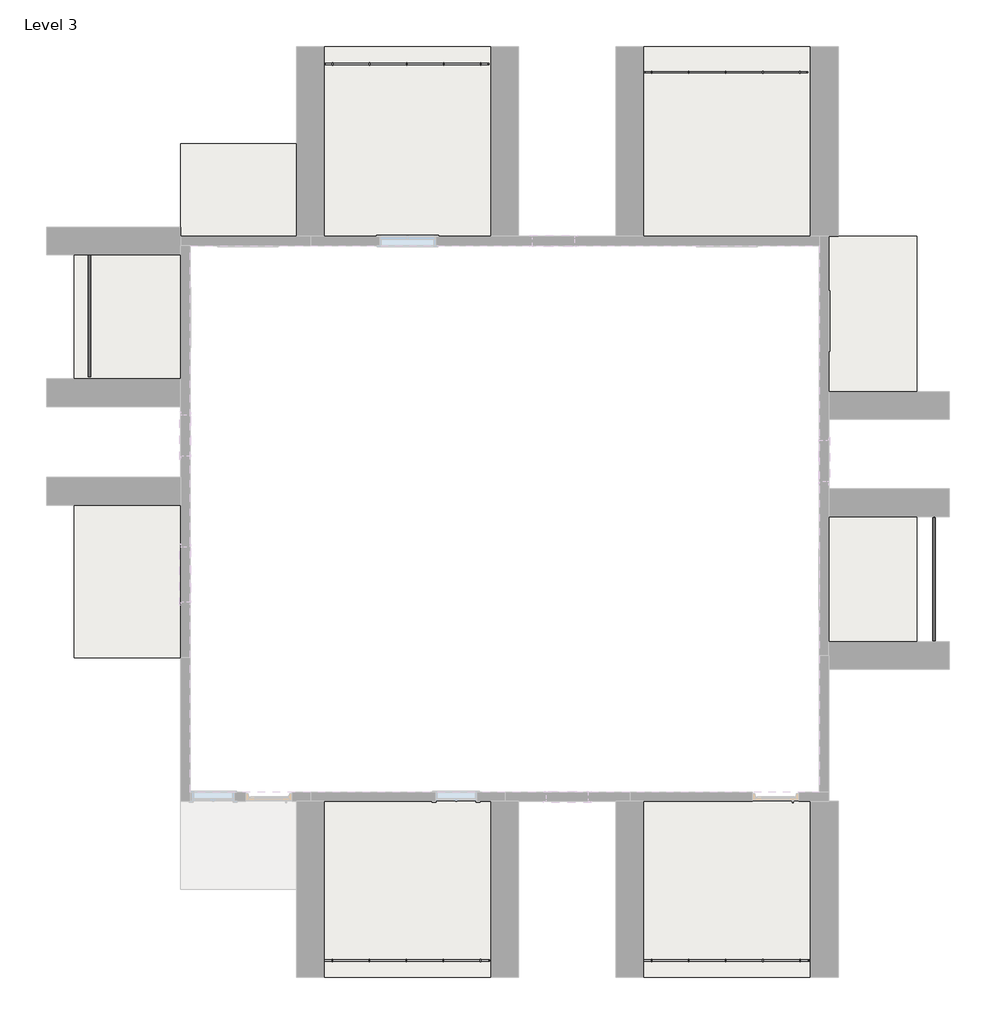
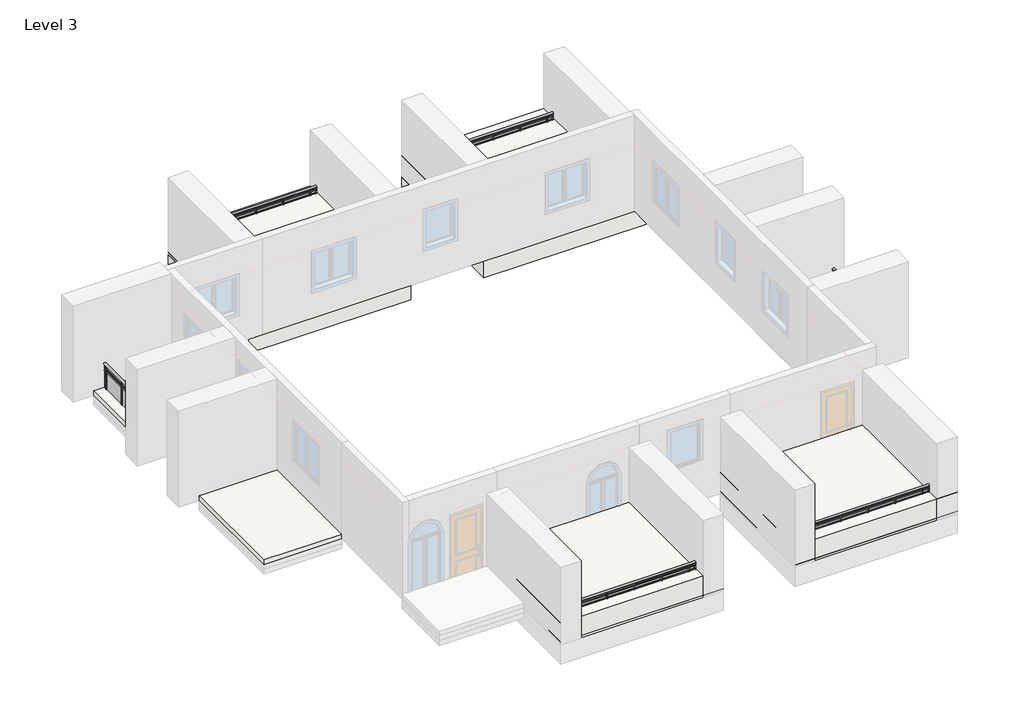
# One storey, part 2 of 2: 6 railings, 5 slabs.
"""IFC4 building model written with IfcOpenShell, lengths in millimetres."""

from ifc_helpers import new_model, si_unit, point, frame, origin, place, context, project, spatial, polyline, ellipse_curve, trimmed, outline, extrude, element, save
from ifc_brep_helpers import plane_surface, extruded_surface, advanced_brep

model = new_model("IFC4")

# Units and contexts
model_context = context("Model", 3, world=origin())
ifc_project = project(units=[si_unit("LENGTHUNIT", "METRE", prefix="MILLI")], contexts=[model_context])

# Site, building, storey
site = spatial("IfcSite", under=ifc_project)
building = spatial("IfcBuilding", under=site)
storey = spatial("IfcBuildingStorey", under=building, Name="Level 3", Elevation=6096.0)

# Railings
placement = place(None, origin())
element("IfcRailing", 1, ObjectType="Glass Panel - Bottom Fill", at=placement, inside=storey, context=model_context, shape_type="SolidModel", body=[
    advanced_brep(
    [(-9258.4937431, -9324.2034265, 7315.2), (-9258.4937431, -9400.4034265, 7315.2), (-5600.8937431, -9324.2034265, 7315.2), (-5600.8937431, -9400.4034265, 7315.2)],
    [
        (0, 1, ellipse_curve(frame((-9258.4937431, -9362.3034265, 7315.2), z_axis=(-1.0, 0.0, 0.0), x_axis=(0.0, -1.0, 0.0)), 38.1, 28.575)),
        (1, 0, ellipse_curve(frame((-9258.4937431, -9362.3034265, 7315.2), z_axis=(-1.0, 0.0, 0.0), x_axis=(0.0, -1.0, 0.0)), 38.1, 28.575)),
        (2, 3, ellipse_curve(frame((-5600.8937431, -9362.3034265, 7315.2), z_axis=(1.0, 0.0, 0.0), x_axis=(0.0, -1.0, 0.0)), 38.1, 28.575)),
        (3, 2, ellipse_curve(frame((-5600.8937431, -9362.3034265, 7315.2), z_axis=(1.0, 0.0, 0.0), x_axis=(0.0, -1.0, 0.0)), 38.1, 28.575)),
        (0, 2),
        (3, 1),
    ],
    [
        plane_surface(frame((-9258.4937431, -9362.3034265, 7315.2), z_axis=(-1.0, 0.0, 0.0), x_axis=(0.0, 1.0, 0.0))),
        plane_surface(frame((-5600.8937431, -9362.3034265, 7315.2), z_axis=(1.0, 0.0, 0.0), x_axis=(0.0, 1.0, 0.0))),
        extruded_surface(trimmed(ellipse_curve(frame((-5600.8937431, -9362.3034265, 7315.2), z_axis=(-1.0, 0.0, 0.0), x_axis=(0.0, -1.0, 0.0)), 38.1, 28.575), [point((-5600.8937431, -9324.2034265, 7315.2))], [point((-5600.8937431, -9400.4034265, 7315.2))], True, "CARTESIAN"), (-3657.5999999999995, 0.0, 0.0), 3657.5999999999995),
        extruded_surface(trimmed(ellipse_curve(frame((-5600.8937431, -9362.3034265, 7315.2), z_axis=(-1.0, 0.0, 0.0), x_axis=(0.0, -1.0, 0.0)), 38.1, 28.575), [point((-5600.8937431, -9400.4034265, 7315.2))], [point((-5600.8937431, -9324.2034265, 7315.2))], True, "CARTESIAN"), (-3657.5999999999995, 0.0, 0.0), 3657.5999999999995),
    ],
    [
        (0, [[1, 2]]),
        (1, [[3, 4]]),
        (2, [[-1, 5, -4, 6]]),
        (3, [[-2, -6, -3, -5]]),
    ],
),
    extrude(outline(polyline([(-9258.4937431, -9375.0034265), (-9258.4937431, -9349.6034265), (-5600.8937431, -9349.6034265), (-5600.8937431, -9375.0034265), (-9258.4937431, -9375.0034265)])), frame((0.0, 0.0, 7200.9), z_axis=(0.0, 0.0, 1.0), x_axis=(1.0, 0.0, 0.0)), (0.0, 0.0, 1.0), 25.4),
    extrude(outline(polyline([(-9258.4937431, -9375.0034265), (-9258.4937431, -9349.6034265), (-5600.8937431, -9349.6034265), (-5600.8937431, -9375.0034265), (-9258.4937431, -9375.0034265)])), frame((0.0, 0.0, 7099.3), z_axis=(0.0, 0.0, 1.0), x_axis=(1.0, 0.0, 0.0)), (0.0, 0.0, 1.0), 25.4),
    extrude(outline(polyline([(-5810.4437431, -9387.7034265), (-5810.4437431, -9336.9034265), (-5797.7437431, -9336.9034265), (-5797.7437431, -9387.7034265), (-5810.4437431, -9387.7034265)])), frame((0.0, 0.0, 6400.8), z_axis=(0.0, 0.0, 1.0), x_axis=(1.0, 0.0, 0.0)), (0.0, 0.0, 1.0), 885.6788223),
    extrude(outline(polyline([(-6616.8937431, -9355.7682695), (-5804.0937431, -9355.7682695), (-5804.0937431, -9362.1182695), (-6616.8937431, -9362.1182695), (-6616.8937431, -9355.7682695)])), frame((0.0, 0.0, 6502.4), z_axis=(0.0, 0.0, 1.0), x_axis=(1.0, 0.0, 0.0)), (0.0, 0.0, 1.0), 596.9),
    extrude(outline(polyline([(-6623.2437431, -9387.7034265), (-6623.2437431, -9336.9034265), (-6610.5437431, -9336.9034265), (-6610.5437431, -9387.7034265), (-6623.2437431, -9387.7034265)])), frame((0.0, 0.0, 6400.8), z_axis=(0.0, 0.0, 1.0), x_axis=(1.0, 0.0, 0.0)), (0.0, 0.0, 1.0), 885.6788223),
    extrude(outline(polyline([(-7429.6937431, -9355.7682695), (-6616.8937431, -9355.7682695), (-6616.8937431, -9362.1182695), (-7429.6937431, -9362.1182695), (-7429.6937431, -9355.7682695)])), frame((0.0, 0.0, 6502.4), z_axis=(0.0, 0.0, 1.0), x_axis=(1.0, 0.0, 0.0)), (0.0, 0.0, 1.0), 596.9),
    extrude(outline(polyline([(-7436.0437431, -9387.7034265), (-7436.0437431, -9336.9034265), (-7423.3437431, -9336.9034265), (-7423.3437431, -9387.7034265), (-7436.0437431, -9387.7034265)])), frame((0.0, 0.0, 6400.8), z_axis=(0.0, 0.0, 1.0), x_axis=(1.0, 0.0, 0.0)), (0.0, 0.0, 1.0), 885.6788223),
    extrude(outline(polyline([(-8242.4937431, -9355.7682695), (-7429.6937431, -9355.7682695), (-7429.6937431, -9362.1182695), (-8242.4937431, -9362.1182695), (-8242.4937431, -9355.7682695)])), frame((0.0, 0.0, 6502.4), z_axis=(0.0, 0.0, 1.0), x_axis=(1.0, 0.0, 0.0)), (0.0, 0.0, 1.0), 596.9),
    extrude(outline(polyline([(-8248.8437431, -9387.7034265), (-8248.8437431, -9336.9034265), (-8236.1437431, -9336.9034265), (-8236.1437431, -9387.7034265), (-8248.8437431, -9387.7034265)])), frame((0.0, 0.0, 6400.8), z_axis=(0.0, 0.0, 1.0), x_axis=(1.0, 0.0, 0.0)), (0.0, 0.0, 1.0), 885.6788223),
    extrude(outline(polyline([(-9055.2937431, -9355.7682695), (-8242.4937431, -9355.7682695), (-8242.4937431, -9362.1182695), (-9055.2937431, -9362.1182695), (-9055.2937431, -9355.7682695)])), frame((0.0, 0.0, 6502.4), z_axis=(0.0, 0.0, 1.0), x_axis=(1.0, 0.0, 0.0)), (0.0, 0.0, 1.0), 596.9),
    extrude(outline(polyline([(-9061.6437431, -9387.7034265), (-9061.6437431, -9336.9034265), (-9048.9437431, -9336.9034265), (-9048.9437431, -9387.7034265), (-9061.6437431, -9387.7034265)])), frame((0.0, 0.0, 6400.8), z_axis=(0.0, 0.0, 1.0), x_axis=(1.0, 0.0, 0.0)), (0.0, 0.0, 1.0), 885.6788223),
    extrude(outline(polyline([(-5613.5937431, -9371.8284265), (-5613.5937431, -9352.7784265), (-5594.5437431, -9352.7784265), (-5594.5437431, -9371.8284265), (-5613.5937431, -9371.8284265)])), frame((0.0, 0.0, 6400.8), z_axis=(0.0, 0.0, 1.0), x_axis=(1.0, 0.0, 0.0)), (0.0, 0.0, 1.0), 885.6788223),
    extrude(outline(polyline([(-9264.8437431, -9371.8284265), (-9264.8437431, -9352.7784265), (-9245.7937431, -9352.7784265), (-9245.7937431, -9371.8284265), (-9264.8437431, -9371.8284265)])), frame((0.0, 0.0, 6400.8), z_axis=(0.0, 0.0, 1.0), x_axis=(1.0, 0.0, 0.0)), (0.0, 0.0, 1.0), 885.6788223),
])
element("IfcRailing", 2, ObjectType="Glass Panel - Bottom Fill", at=placement, inside=storey, context=model_context, shape_type="SolidModel", body=[
    advanced_brep(
    [(-2248.0325613, -9324.2034265, 7310.1393423), (-2248.0325613, -9400.4034265, 7310.1393423), (1409.5674387, -9324.2034265, 7310.1393423), (1409.5674387, -9400.4034265, 7310.1393423)],
    [
        (0, 1, ellipse_curve(frame((-2248.0325613, -9362.3034265, 7310.1393423), z_axis=(-1.0, 0.0, 0.0), x_axis=(0.0, -1.0, 0.0)), 38.1, 28.575)),
        (1, 0, ellipse_curve(frame((-2248.0325613, -9362.3034265, 7310.1393423), z_axis=(-1.0, 0.0, 0.0), x_axis=(0.0, -1.0, 0.0)), 38.1, 28.575)),
        (2, 3, ellipse_curve(frame((1409.5674387, -9362.3034265, 7310.1393423), z_axis=(1.0, 0.0, 0.0), x_axis=(0.0, -1.0, 0.0)), 38.1, 28.575)),
        (3, 2, ellipse_curve(frame((1409.5674387, -9362.3034265, 7310.1393423), z_axis=(1.0, 0.0, 0.0), x_axis=(0.0, -1.0, 0.0)), 38.1, 28.575)),
        (0, 2),
        (3, 1),
    ],
    [
        plane_surface(frame((-2248.0325613, -9362.3034265, 7310.1393423), z_axis=(-1.0, 0.0, 0.0), x_axis=(0.0, 1.0, 0.0))),
        plane_surface(frame((1409.5674387, -9362.3034265, 7310.1393423), z_axis=(1.0, 0.0, 0.0), x_axis=(0.0, 1.0, 0.0))),
        extruded_surface(trimmed(ellipse_curve(frame((1409.5674387, -9362.3034265, 7310.1393423), z_axis=(-1.0, 0.0, 0.0), x_axis=(0.0, -1.0, 0.0)), 38.1, 28.575), [point((1409.5674387, -9324.2034265, 7310.1393423))], [point((1409.5674387, -9400.4034265, 7310.1393423))], True, "CARTESIAN"), (-3657.6, 0.0, 0.0), 3657.6),
        extruded_surface(trimmed(ellipse_curve(frame((1409.5674387, -9362.3034265, 7310.1393423), z_axis=(-1.0, 0.0, 0.0), x_axis=(0.0, -1.0, 0.0)), 38.1, 28.575), [point((1409.5674387, -9400.4034265, 7310.1393423))], [point((1409.5674387, -9324.2034265, 7310.1393423))], True, "CARTESIAN"), (-3657.6, 0.0, 0.0), 3657.6),
    ],
    [
        (0, [[1, 2]]),
        (1, [[3, 4]]),
        (2, [[-1, 5, -4, 6]]),
        (3, [[-2, -6, -3, -5]]),
    ],
),
    extrude(outline(polyline([(-2248.0325613, -9375.0034265), (-2248.0325613, -9349.6034265), (1409.5674387, -9349.6034265), (1409.5674387, -9375.0034265), (-2248.0325613, -9375.0034265)])), frame((0.0, 0.0, 7195.8393423), z_axis=(0.0, 0.0, 1.0), x_axis=(1.0, 0.0, 0.0)), (0.0, 0.0, 1.0), 25.4),
    extrude(outline(polyline([(-2248.0325613, -9375.0034265), (-2248.0325613, -9349.6034265), (1409.5674387, -9349.6034265), (1409.5674387, -9375.0034265), (-2248.0325613, -9375.0034265)])), frame((0.0, 0.0, 7094.2393423), z_axis=(0.0, 0.0, 1.0), x_axis=(1.0, 0.0, 0.0)), (0.0, 0.0, 1.0), 25.4),
    extrude(outline(polyline([(1200.0174387, -9387.7034265), (1200.0174387, -9336.9034265), (1212.7174387, -9336.9034265), (1212.7174387, -9387.7034265), (1200.0174387, -9387.7034265)])), frame((0.0, 0.0, 6395.7393423), z_axis=(0.0, 0.0, 1.0), x_axis=(1.0, 0.0, 0.0)), (0.0, 0.0, 1.0), 885.6788223),
    extrude(outline(polyline([(393.5674387, -9355.7682695), (1206.3674387, -9355.7682695), (1206.3674387, -9362.1182695), (393.5674387, -9362.1182695), (393.5674387, -9355.7682695)])), frame((0.0, 0.0, 6497.3393423), z_axis=(0.0, 0.0, 1.0), x_axis=(1.0, 0.0, 0.0)), (0.0, 0.0, 1.0), 596.9),
    extrude(outline(polyline([(387.2174387, -9387.7034265), (387.2174387, -9336.9034265), (399.9174387, -9336.9034265), (399.9174387, -9387.7034265), (387.2174387, -9387.7034265)])), frame((0.0, 0.0, 6395.7393423), z_axis=(0.0, 0.0, 1.0), x_axis=(1.0, 0.0, 0.0)), (0.0, 0.0, 1.0), 885.6788223),
    extrude(outline(polyline([(-419.2325613, -9355.7682695), (393.5674387, -9355.7682695), (393.5674387, -9362.1182695), (-419.2325613, -9362.1182695), (-419.2325613, -9355.7682695)])), frame((0.0, 0.0, 6497.3393423), z_axis=(0.0, 0.0, 1.0), x_axis=(1.0, 0.0, 0.0)), (0.0, 0.0, 1.0), 596.9),
    extrude(outline(polyline([(-425.5825613, -9387.7034265), (-425.5825613, -9336.9034265), (-412.8825613, -9336.9034265), (-412.8825613, -9387.7034265), (-425.5825613, -9387.7034265)])), frame((0.0, 0.0, 6395.7393423), z_axis=(0.0, 0.0, 1.0), x_axis=(1.0, 0.0, 0.0)), (0.0, 0.0, 1.0), 885.6788223),
    extrude(outline(polyline([(-1232.0325613, -9355.7682695), (-419.2325613, -9355.7682695), (-419.2325613, -9362.1182695), (-1232.0325613, -9362.1182695), (-1232.0325613, -9355.7682695)])), frame((0.0, 0.0, 6497.3393423), z_axis=(0.0, 0.0, 1.0), x_axis=(1.0, 0.0, 0.0)), (0.0, 0.0, 1.0), 596.9),
    extrude(outline(polyline([(-1238.3825613, -9387.7034265), (-1238.3825613, -9336.9034265), (-1225.6825613, -9336.9034265), (-1225.6825613, -9387.7034265), (-1238.3825613, -9387.7034265)])), frame((0.0, 0.0, 6395.7393423), z_axis=(0.0, 0.0, 1.0), x_axis=(1.0, 0.0, 0.0)), (0.0, 0.0, 1.0), 885.6788223),
    extrude(outline(polyline([(-2044.8325613, -9355.7682695), (-1232.0325613, -9355.7682695), (-1232.0325613, -9362.1182695), (-2044.8325613, -9362.1182695), (-2044.8325613, -9355.7682695)])), frame((0.0, 0.0, 6497.3393423), z_axis=(0.0, 0.0, 1.0), x_axis=(1.0, 0.0, 0.0)), (0.0, 0.0, 1.0), 596.9),
    extrude(outline(polyline([(-2051.1825613, -9387.7034265), (-2051.1825613, -9336.9034265), (-2038.4825613, -9336.9034265), (-2038.4825613, -9387.7034265), (-2051.1825613, -9387.7034265)])), frame((0.0, 0.0, 6395.7393423), z_axis=(0.0, 0.0, 1.0), x_axis=(1.0, 0.0, 0.0)), (0.0, 0.0, 1.0), 885.6788223),
    extrude(outline(polyline([(1396.8674387, -9371.8284265), (1396.8674387, -9352.7784265), (1415.9174387, -9352.7784265), (1415.9174387, -9371.8284265), (1396.8674387, -9371.8284265)])), frame((0.0, 0.0, 6395.7393423), z_axis=(0.0, 0.0, 1.0), x_axis=(1.0, 0.0, 0.0)), (0.0, 0.0, 1.0), 885.6788223),
    extrude(outline(polyline([(-2254.3825613, -9371.8284265), (-2254.3825613, -9352.7784265), (-2235.3325613, -9352.7784265), (-2235.3325613, -9371.8284265), (-2254.3825613, -9371.8284265)])), frame((0.0, 0.0, 6395.7393423), z_axis=(0.0, 0.0, 1.0), x_axis=(1.0, 0.0, 0.0)), (0.0, 0.0, 1.0), 885.6788223),
])
element("IfcRailing", 3, ObjectType="Glass Panel - Bottom Fill", at=placement, inside=storey, context=model_context, shape_type="SolidModel", body=[
    advanced_brep(
    [(-14351.1937431, 6115.813611, 7315.2), (-14427.3937431, 6115.813611, 7315.2), (-14351.1937431, 3448.813611, 7315.2), (-14427.3937431, 3448.813611, 7315.2)],
    [
        (0, 1, ellipse_curve(frame((-14389.2937431, 6115.813611, 7315.2), z_axis=(0.0, 1.0, 0.0), x_axis=(-1.0, 0.0, 0.0)), 38.1, 28.575)),
        (1, 0, ellipse_curve(frame((-14389.2937431, 6115.813611, 7315.2), z_axis=(0.0, 1.0, 0.0), x_axis=(-1.0, 0.0, 0.0)), 38.1, 28.575)),
        (2, 3, ellipse_curve(frame((-14389.2937431, 3448.813611, 7315.2), z_axis=(0.0, -1.0, 0.0), x_axis=(-1.0, 0.0, 0.0)), 38.1, 28.575)),
        (3, 2, ellipse_curve(frame((-14389.2937431, 3448.813611, 7315.2), z_axis=(0.0, -1.0, 0.0), x_axis=(-1.0, 0.0, 0.0)), 38.1, 28.575)),
        (0, 2),
        (3, 1),
    ],
    [
        plane_surface(frame((-14389.2937431, 6115.813611, 7315.2), z_axis=(0.0, 1.0, 0.0), x_axis=(0.0, 0.0, -1.0))),
        plane_surface(frame((-14389.2937431, 3448.813611, 7315.2), z_axis=(0.0, -1.0, 0.0), x_axis=(0.0, 0.0, -1.0))),
        extruded_surface(trimmed(ellipse_curve(frame((-14389.2937431, 3448.813611, 7315.2), z_axis=(0.0, 1.0, 0.0), x_axis=(-1.0, 0.0, 0.0)), 38.1, 28.575), [point((-14351.1937431, 3448.813611, 7315.2))], [point((-14427.3937431, 3448.813611, 7315.2))], True, "CARTESIAN"), (0.0, 2666.9999999999995, 0.0), 2666.9999999999995),
        extruded_surface(trimmed(ellipse_curve(frame((-14389.2937431, 3448.813611, 7315.2), z_axis=(0.0, 1.0, 0.0), x_axis=(-1.0, 0.0, 0.0)), 38.1, 28.575), [point((-14427.3937431, 3448.813611, 7315.2))], [point((-14351.1937431, 3448.813611, 7315.2))], True, "CARTESIAN"), (0.0, 2666.9999999999995, 0.0), 2666.9999999999995),
    ],
    [
        (0, [[1, 2]]),
        (1, [[3, 4]]),
        (2, [[-1, 5, -4, 6]]),
        (3, [[-2, -6, -3, -5]]),
    ],
),
    extrude(outline(polyline([(-14401.9937431, 6115.813611), (-14376.5937431, 6115.813611), (-14376.5937431, 3448.813611), (-14401.9937431, 3448.813611), (-14401.9937431, 6115.813611)])), frame((0.0, 0.0, 7200.9), z_axis=(0.0, 0.0, 1.0), x_axis=(1.0, 0.0, 0.0)), (0.0, 0.0, 1.0), 25.4),
    extrude(outline(polyline([(-14401.9937431, 6115.813611), (-14376.5937431, 6115.813611), (-14376.5937431, 3448.813611), (-14401.9937431, 3448.813611), (-14401.9937431, 6115.813611)])), frame((0.0, 0.0, 7099.3), z_axis=(0.0, 0.0, 1.0), x_axis=(1.0, 0.0, 0.0)), (0.0, 0.0, 1.0), 25.4),
    extrude(outline(polyline([(-14414.6937431, 3569.463611), (-14363.8937431, 3569.463611), (-14363.8937431, 3556.763611), (-14414.6937431, 3556.763611), (-14414.6937431, 3569.463611)])), frame((0.0, 0.0, 6400.8), z_axis=(0.0, 0.0, 1.0), x_axis=(1.0, 0.0, 0.0)), (0.0, 0.0, 1.0), 885.6788223),
    extrude(outline(polyline([(-14382.7585861, 4375.913611), (-14382.7585861, 3563.113611), (-14389.1085861, 3563.113611), (-14389.1085861, 4375.913611), (-14382.7585861, 4375.913611)])), frame((0.0, 0.0, 6502.4), z_axis=(0.0, 0.0, 1.0), x_axis=(1.0, 0.0, 0.0)), (0.0, 0.0, 1.0), 596.9),
    extrude(outline(polyline([(-14414.6937431, 4382.263611), (-14363.8937431, 4382.263611), (-14363.8937431, 4369.563611), (-14414.6937431, 4369.563611), (-14414.6937431, 4382.263611)])), frame((0.0, 0.0, 6400.8), z_axis=(0.0, 0.0, 1.0), x_axis=(1.0, 0.0, 0.0)), (0.0, 0.0, 1.0), 885.6788223),
    extrude(outline(polyline([(-14382.7585861, 5188.713611), (-14382.7585861, 4375.913611), (-14389.1085861, 4375.913611), (-14389.1085861, 5188.713611), (-14382.7585861, 5188.713611)])), frame((0.0, 0.0, 6502.4), z_axis=(0.0, 0.0, 1.0), x_axis=(1.0, 0.0, 0.0)), (0.0, 0.0, 1.0), 596.9),
    extrude(outline(polyline([(-14414.6937431, 5195.063611), (-14363.8937431, 5195.063611), (-14363.8937431, 5182.363611), (-14414.6937431, 5182.363611), (-14414.6937431, 5195.063611)])), frame((0.0, 0.0, 6400.8), z_axis=(0.0, 0.0, 1.0), x_axis=(1.0, 0.0, 0.0)), (0.0, 0.0, 1.0), 885.6788223),
    extrude(outline(polyline([(-14382.7585861, 6001.513611), (-14382.7585861, 5188.713611), (-14389.1085861, 5188.713611), (-14389.1085861, 6001.513611), (-14382.7585861, 6001.513611)])), frame((0.0, 0.0, 6502.4), z_axis=(0.0, 0.0, 1.0), x_axis=(1.0, 0.0, 0.0)), (0.0, 0.0, 1.0), 596.9),
    extrude(outline(polyline([(-14414.6937431, 6007.863611), (-14363.8937431, 6007.863611), (-14363.8937431, 5995.163611), (-14414.6937431, 5995.163611), (-14414.6937431, 6007.863611)])), frame((0.0, 0.0, 6400.8), z_axis=(0.0, 0.0, 1.0), x_axis=(1.0, 0.0, 0.0)), (0.0, 0.0, 1.0), 885.6788223),
    extrude(outline(polyline([(-14398.8187431, 3461.513611), (-14379.7687431, 3461.513611), (-14379.7687431, 3442.463611), (-14398.8187431, 3442.463611), (-14398.8187431, 3461.513611)])), frame((0.0, 0.0, 6400.8), z_axis=(0.0, 0.0, 1.0), x_axis=(1.0, 0.0, 0.0)), (0.0, 0.0, 1.0), 885.6788223),
    extrude(outline(polyline([(-14398.8187431, 6122.163611), (-14379.7687431, 6122.163611), (-14379.7687431, 6103.113611), (-14398.8187431, 6103.113611), (-14398.8187431, 6122.163611)])), frame((0.0, 0.0, 6400.8), z_axis=(0.0, 0.0, 1.0), x_axis=(1.0, 0.0, 0.0)), (0.0, 0.0, 1.0), 885.6788223),
])
element("IfcRailing", 4, ObjectType="Glass Panel - Bottom Fill", at=placement, inside=storey, context=model_context, shape_type="SolidModel", body=[
    advanced_brep(
    [(-9229.0758442, 10344.5205237, 7315.2), (-9229.0758442, 10268.3205237, 7315.2), (-5622.2758442, 10344.5205237, 7315.2), (-5622.2758442, 10268.3205237, 7315.2)],
    [
        (0, 1, ellipse_curve(frame((-9229.0758442, 10306.4205237, 7315.2), z_axis=(-1.0, 0.0, 0.0), x_axis=(0.0, -1.0, 0.0)), 38.1, 28.575)),
        (1, 0, ellipse_curve(frame((-9229.0758442, 10306.4205237, 7315.2), z_axis=(-1.0, 0.0, 0.0), x_axis=(0.0, -1.0, 0.0)), 38.1, 28.575)),
        (2, 3, ellipse_curve(frame((-5622.2758442, 10306.4205237, 7315.2), z_axis=(1.0, 0.0, 0.0), x_axis=(0.0, -1.0, 0.0)), 38.1, 28.575)),
        (3, 2, ellipse_curve(frame((-5622.2758442, 10306.4205237, 7315.2), z_axis=(1.0, 0.0, 0.0), x_axis=(0.0, -1.0, 0.0)), 38.1, 28.575)),
        (0, 2),
        (3, 1),
    ],
    [
        plane_surface(frame((-9229.0758442, 10306.4205237, 7315.2), z_axis=(-1.0, 0.0, 0.0), x_axis=(0.0, 1.0, 0.0))),
        plane_surface(frame((-5622.2758442, 10306.4205237, 7315.2), z_axis=(1.0, 0.0, 0.0), x_axis=(0.0, 1.0, 0.0))),
        extruded_surface(trimmed(ellipse_curve(frame((-5622.2758442, 10306.4205237, 7315.2), z_axis=(-1.0, 0.0, 0.0), x_axis=(0.0, -1.0, 0.0)), 38.1, 28.575), [point((-5622.2758442, 10344.5205237, 7315.2))], [point((-5622.2758442, 10268.3205237, 7315.2))], True, "CARTESIAN"), (-3606.8, 0.0, 0.0), 3606.8),
        extruded_surface(trimmed(ellipse_curve(frame((-5622.2758442, 10306.4205237, 7315.2), z_axis=(-1.0, 0.0, 0.0), x_axis=(0.0, -1.0, 0.0)), 38.1, 28.575), [point((-5622.2758442, 10268.3205237, 7315.2))], [point((-5622.2758442, 10344.5205237, 7315.2))], True, "CARTESIAN"), (-3606.8, 0.0, 0.0), 3606.8),
    ],
    [
        (0, [[1, 2]]),
        (1, [[3, 4]]),
        (2, [[-1, 5, -4, 6]]),
        (3, [[-2, -6, -3, -5]]),
    ],
),
    extrude(outline(polyline([(-9229.0758442, 10293.7205237), (-9229.0758442, 10319.1205237), (-5622.2758442, 10319.1205237), (-5622.2758442, 10293.7205237), (-9229.0758442, 10293.7205237)])), frame((0.0, 0.0, 7200.9), z_axis=(0.0, 0.0, 1.0), x_axis=(1.0, 0.0, 0.0)), (0.0, 0.0, 1.0), 25.4),
    extrude(outline(polyline([(-9229.0758442, 10293.7205237), (-9229.0758442, 10319.1205237), (-5622.2758442, 10319.1205237), (-5622.2758442, 10293.7205237), (-9229.0758442, 10293.7205237)])), frame((0.0, 0.0, 7099.3), z_axis=(0.0, 0.0, 1.0), x_axis=(1.0, 0.0, 0.0)), (0.0, 0.0, 1.0), 25.4),
    extrude(outline(polyline([(-5806.4258442, 10281.0205237), (-5806.4258442, 10331.8205237), (-5793.7258442, 10331.8205237), (-5793.7258442, 10281.0205237), (-5806.4258442, 10281.0205237)])), frame((0.0, 0.0, 6400.8), z_axis=(0.0, 0.0, 1.0), x_axis=(1.0, 0.0, 0.0)), (0.0, 0.0, 1.0), 885.6788223),
    extrude(outline(polyline([(-6612.8758442, 10312.9556807), (-5800.0758442, 10312.9556807), (-5800.0758442, 10306.6056807), (-6612.8758442, 10306.6056807), (-6612.8758442, 10312.9556807)])), frame((0.0, 0.0, 6502.4), z_axis=(0.0, 0.0, 1.0), x_axis=(1.0, 0.0, 0.0)), (0.0, 0.0, 1.0), 596.9),
    extrude(outline(polyline([(-6619.2258442, 10281.0205237), (-6619.2258442, 10331.8205237), (-6606.5258442, 10331.8205237), (-6606.5258442, 10281.0205237), (-6619.2258442, 10281.0205237)])), frame((0.0, 0.0, 6400.8), z_axis=(0.0, 0.0, 1.0), x_axis=(1.0, 0.0, 0.0)), (0.0, 0.0, 1.0), 885.6788223),
    extrude(outline(polyline([(-7425.6758442, 10312.9556807), (-6612.8758442, 10312.9556807), (-6612.8758442, 10306.6056807), (-7425.6758442, 10306.6056807), (-7425.6758442, 10312.9556807)])), frame((0.0, 0.0, 6502.4), z_axis=(0.0, 0.0, 1.0), x_axis=(1.0, 0.0, 0.0)), (0.0, 0.0, 1.0), 596.9),
    extrude(outline(polyline([(-7432.0258442, 10281.0205237), (-7432.0258442, 10331.8205237), (-7419.3258442, 10331.8205237), (-7419.3258442, 10281.0205237), (-7432.0258442, 10281.0205237)])), frame((0.0, 0.0, 6400.8), z_axis=(0.0, 0.0, 1.0), x_axis=(1.0, 0.0, 0.0)), (0.0, 0.0, 1.0), 885.6788223),
    extrude(outline(polyline([(-8238.4758442, 10312.9556807), (-7425.6758442, 10312.9556807), (-7425.6758442, 10306.6056807), (-8238.4758442, 10306.6056807), (-8238.4758442, 10312.9556807)])), frame((0.0, 0.0, 6502.4), z_axis=(0.0, 0.0, 1.0), x_axis=(1.0, 0.0, 0.0)), (0.0, 0.0, 1.0), 596.9),
    extrude(outline(polyline([(-8244.8258442, 10281.0205237), (-8244.8258442, 10331.8205237), (-8232.1258442, 10331.8205237), (-8232.1258442, 10281.0205237), (-8244.8258442, 10281.0205237)])), frame((0.0, 0.0, 6400.8), z_axis=(0.0, 0.0, 1.0), x_axis=(1.0, 0.0, 0.0)), (0.0, 0.0, 1.0), 885.6788223),
    extrude(outline(polyline([(-9051.2758442, 10312.9556807), (-8238.4758442, 10312.9556807), (-8238.4758442, 10306.6056807), (-9051.2758442, 10306.6056807), (-9051.2758442, 10312.9556807)])), frame((0.0, 0.0, 6502.4), z_axis=(0.0, 0.0, 1.0), x_axis=(1.0, 0.0, 0.0)), (0.0, 0.0, 1.0), 596.9),
    extrude(outline(polyline([(-9057.6258442, 10281.0205237), (-9057.6258442, 10331.8205237), (-9044.9258442, 10331.8205237), (-9044.9258442, 10281.0205237), (-9057.6258442, 10281.0205237)])), frame((0.0, 0.0, 6400.8), z_axis=(0.0, 0.0, 1.0), x_axis=(1.0, 0.0, 0.0)), (0.0, 0.0, 1.0), 885.6788223),
    extrude(outline(polyline([(-5634.9758442, 10296.8955237), (-5634.9758442, 10315.9455237), (-5615.9258442, 10315.9455237), (-5615.9258442, 10296.8955237), (-5634.9758442, 10296.8955237)])), frame((0.0, 0.0, 6400.8), z_axis=(0.0, 0.0, 1.0), x_axis=(1.0, 0.0, 0.0)), (0.0, 0.0, 1.0), 885.6788223),
    extrude(outline(polyline([(-9235.4258442, 10296.8955237), (-9235.4258442, 10315.9455237), (-9216.3758442, 10315.9455237), (-9216.3758442, 10296.8955237), (-9235.4258442, 10296.8955237)])), frame((0.0, 0.0, 6400.8), z_axis=(0.0, 0.0, 1.0), x_axis=(1.0, 0.0, 0.0)), (0.0, 0.0, 1.0), 885.6788223),
])
element("IfcRailing", 5, ObjectType="Glass Panel - Bottom Fill", at=placement, inside=storey, context=model_context, shape_type="SolidModel", body=[
    advanced_brep(
    [(-2210.3891352, 10161.3373193, 7315.2), (-2210.3891352, 10085.1373193, 7315.2), (1371.0108648, 10161.3373193, 7315.2), (1371.0108648, 10085.1373193, 7315.2)],
    [
        (0, 1, ellipse_curve(frame((-2210.3891352, 10123.2373193, 7315.2), z_axis=(-1.0, 0.0, 0.0), x_axis=(0.0, -1.0, 0.0)), 38.1, 28.575)),
        (1, 0, ellipse_curve(frame((-2210.3891352, 10123.2373193, 7315.2), z_axis=(-1.0, 0.0, 0.0), x_axis=(0.0, -1.0, 0.0)), 38.1, 28.575)),
        (2, 3, ellipse_curve(frame((1371.0108648, 10123.2373193, 7315.2), z_axis=(1.0, 0.0, 0.0), x_axis=(0.0, -1.0, 0.0)), 38.1, 28.575)),
        (3, 2, ellipse_curve(frame((1371.0108648, 10123.2373193, 7315.2), z_axis=(1.0, 0.0, 0.0), x_axis=(0.0, -1.0, 0.0)), 38.1, 28.575)),
        (0, 2),
        (3, 1),
    ],
    [
        plane_surface(frame((-2210.3891352, 10123.2373193, 7315.2), z_axis=(-1.0, 0.0, 0.0), x_axis=(0.0, 1.0, 0.0))),
        plane_surface(frame((1371.0108648, 10123.2373193, 7315.2), z_axis=(1.0, 0.0, 0.0), x_axis=(0.0, 1.0, 0.0))),
        extruded_surface(trimmed(ellipse_curve(frame((1371.0108648, 10123.2373193, 7315.2), z_axis=(-1.0, 0.0, 0.0), x_axis=(0.0, -1.0, 0.0)), 38.1, 28.575), [point((1371.0108648, 10161.3373193, 7315.2))], [point((1371.0108648, 10085.1373193, 7315.2))], True, "CARTESIAN"), (-3581.4, 0.0, 0.0), 3581.4),
        extruded_surface(trimmed(ellipse_curve(frame((1371.0108648, 10123.2373193, 7315.2), z_axis=(-1.0, 0.0, 0.0), x_axis=(0.0, -1.0, 0.0)), 38.1, 28.575), [point((1371.0108648, 10085.1373193, 7315.2))], [point((1371.0108648, 10161.3373193, 7315.2))], True, "CARTESIAN"), (-3581.4, 0.0, 0.0), 3581.4),
    ],
    [
        (0, [[1, 2]]),
        (1, [[3, 4]]),
        (2, [[-1, 5, -4, 6]]),
        (3, [[-2, -6, -3, -5]]),
    ],
),
    extrude(outline(polyline([(-2210.3891352, 10110.5373193), (-2210.3891352, 10135.9373193), (1371.0108648, 10135.9373193), (1371.0108648, 10110.5373193), (-2210.3891352, 10110.5373193)])), frame((0.0, 0.0, 7200.9), z_axis=(0.0, 0.0, 1.0), x_axis=(1.0, 0.0, 0.0)), (0.0, 0.0, 1.0), 25.4),
    extrude(outline(polyline([(-2210.3891352, 10110.5373193), (-2210.3891352, 10135.9373193), (1371.0108648, 10135.9373193), (1371.0108648, 10110.5373193), (-2210.3891352, 10110.5373193)])), frame((0.0, 0.0, 7099.3), z_axis=(0.0, 0.0, 1.0), x_axis=(1.0, 0.0, 0.0)), (0.0, 0.0, 1.0), 25.4),
    extrude(outline(polyline([(1199.5608648, 10097.8373193), (1199.5608648, 10148.6373193), (1212.2608648, 10148.6373193), (1212.2608648, 10097.8373193), (1199.5608648, 10097.8373193)])), frame((0.0, 0.0, 6400.8), z_axis=(0.0, 0.0, 1.0), x_axis=(1.0, 0.0, 0.0)), (0.0, 0.0, 1.0), 885.6788223),
    extrude(outline(polyline([(393.1108648, 10129.7724763), (1205.9108648, 10129.7724763), (1205.9108648, 10123.4224763), (393.1108648, 10123.4224763), (393.1108648, 10129.7724763)])), frame((0.0, 0.0, 6502.4), z_axis=(0.0, 0.0, 1.0), x_axis=(1.0, 0.0, 0.0)), (0.0, 0.0, 1.0), 596.9),
    extrude(outline(polyline([(386.7608648, 10097.8373193), (386.7608648, 10148.6373193), (399.4608648, 10148.6373193), (399.4608648, 10097.8373193), (386.7608648, 10097.8373193)])), frame((0.0, 0.0, 6400.8), z_axis=(0.0, 0.0, 1.0), x_axis=(1.0, 0.0, 0.0)), (0.0, 0.0, 1.0), 885.6788223),
    extrude(outline(polyline([(-419.6891352, 10129.7724763), (393.1108648, 10129.7724763), (393.1108648, 10123.4224763), (-419.6891352, 10123.4224763), (-419.6891352, 10129.7724763)])), frame((0.0, 0.0, 6502.4), z_axis=(0.0, 0.0, 1.0), x_axis=(1.0, 0.0, 0.0)), (0.0, 0.0, 1.0), 596.9),
    extrude(outline(polyline([(-426.0391352, 10097.8373193), (-426.0391352, 10148.6373193), (-413.3391352, 10148.6373193), (-413.3391352, 10097.8373193), (-426.0391352, 10097.8373193)])), frame((0.0, 0.0, 6400.8), z_axis=(0.0, 0.0, 1.0), x_axis=(1.0, 0.0, 0.0)), (0.0, 0.0, 1.0), 885.6788223),
    extrude(outline(polyline([(-1232.4891352, 10129.7724763), (-419.6891352, 10129.7724763), (-419.6891352, 10123.4224763), (-1232.4891352, 10123.4224763), (-1232.4891352, 10129.7724763)])), frame((0.0, 0.0, 6502.4), z_axis=(0.0, 0.0, 1.0), x_axis=(1.0, 0.0, 0.0)), (0.0, 0.0, 1.0), 596.9),
    extrude(outline(polyline([(-1238.8391352, 10097.8373193), (-1238.8391352, 10148.6373193), (-1226.1391352, 10148.6373193), (-1226.1391352, 10097.8373193), (-1238.8391352, 10097.8373193)])), frame((0.0, 0.0, 6400.8), z_axis=(0.0, 0.0, 1.0), x_axis=(1.0, 0.0, 0.0)), (0.0, 0.0, 1.0), 885.6788223),
    extrude(outline(polyline([(-2045.2891352, 10129.7724763), (-1232.4891352, 10129.7724763), (-1232.4891352, 10123.4224763), (-2045.2891352, 10123.4224763), (-2045.2891352, 10129.7724763)])), frame((0.0, 0.0, 6502.4), z_axis=(0.0, 0.0, 1.0), x_axis=(1.0, 0.0, 0.0)), (0.0, 0.0, 1.0), 596.9),
    extrude(outline(polyline([(-2051.6391352, 10097.8373193), (-2051.6391352, 10148.6373193), (-2038.9391352, 10148.6373193), (-2038.9391352, 10097.8373193), (-2051.6391352, 10097.8373193)])), frame((0.0, 0.0, 6400.8), z_axis=(0.0, 0.0, 1.0), x_axis=(1.0, 0.0, 0.0)), (0.0, 0.0, 1.0), 885.6788223),
    extrude(outline(polyline([(1358.3108648, 10113.7123193), (1358.3108648, 10132.7623193), (1377.3608648, 10132.7623193), (1377.3608648, 10113.7123193), (1358.3108648, 10113.7123193)])), frame((0.0, 0.0, 6400.8), z_axis=(0.0, 0.0, 1.0), x_axis=(1.0, 0.0, 0.0)), (0.0, 0.0, 1.0), 885.6788223),
    extrude(outline(polyline([(-2216.7391352, 10113.7123193), (-2216.7391352, 10132.7623193), (-2197.6891352, 10132.7623193), (-2197.6891352, 10113.7123193), (-2216.7391352, 10113.7123193)])), frame((0.0, 0.0, 6400.8), z_axis=(0.0, 0.0, 1.0), x_axis=(1.0, 0.0, 0.0)), (0.0, 0.0, 1.0), 885.6788223),
])
element("IfcRailing", 6, ObjectType="Glass Panel - Bottom Fill", at=placement, inside=storey, context=model_context, shape_type="SolidModel", body=[
    advanced_brep(
    [(4190.8062569, 350.013611, 7315.2), (4114.6062569, 350.013611, 7315.2), (4190.8062569, -2342.386389, 7315.2), (4114.6062569, -2342.386389, 7315.2)],
    [
        (0, 1, ellipse_curve(frame((4152.7062569, 350.013611, 7315.2), z_axis=(0.0, 1.0, 0.0), x_axis=(-1.0, 0.0, 0.0)), 38.1, 28.575)),
        (1, 0, ellipse_curve(frame((4152.7062569, 350.013611, 7315.2), z_axis=(0.0, 1.0, 0.0), x_axis=(-1.0, 0.0, 0.0)), 38.1, 28.575)),
        (2, 3, ellipse_curve(frame((4152.7062569, -2342.386389, 7315.2), z_axis=(0.0, -1.0, 0.0), x_axis=(-1.0, 0.0, 0.0)), 38.1, 28.575)),
        (3, 2, ellipse_curve(frame((4152.7062569, -2342.386389, 7315.2), z_axis=(0.0, -1.0, 0.0), x_axis=(-1.0, 0.0, 0.0)), 38.1, 28.575)),
        (0, 2),
        (3, 1),
    ],
    [
        plane_surface(frame((4152.7062569, 350.013611, 7315.2), z_axis=(0.0, 1.0, 0.0), x_axis=(0.0, 0.0, -1.0))),
        plane_surface(frame((4152.7062569, -2342.386389, 7315.2), z_axis=(0.0, -1.0, 0.0), x_axis=(0.0, 0.0, -1.0))),
        extruded_surface(trimmed(ellipse_curve(frame((4152.7062569, -2342.386389, 7315.2), z_axis=(0.0, 1.0, 0.0), x_axis=(-1.0, 0.0, 0.0)), 38.1, 28.575), [point((4190.8062569, -2342.386389, 7315.2))], [point((4114.6062569, -2342.386389, 7315.2))], True, "CARTESIAN"), (0.0, 2692.3999999999996, 0.0), 2692.3999999999996),
        extruded_surface(trimmed(ellipse_curve(frame((4152.7062569, -2342.386389, 7315.2), z_axis=(0.0, 1.0, 0.0), x_axis=(-1.0, 0.0, 0.0)), 38.1, 28.575), [point((4114.6062569, -2342.386389, 7315.2))], [point((4190.8062569, -2342.386389, 7315.2))], True, "CARTESIAN"), (0.0, 2692.3999999999996, 0.0), 2692.3999999999996),
    ],
    [
        (0, [[1, 2]]),
        (1, [[3, 4]]),
        (2, [[-1, 5, -4, 6]]),
        (3, [[-2, -6, -3, -5]]),
    ],
),
    extrude(outline(polyline([(4140.0062569, 350.013611), (4165.4062569, 350.013611), (4165.4062569, -2342.386389), (4140.0062569, -2342.386389), (4140.0062569, 350.013611)])), frame((0.0, 0.0, 7200.9), z_axis=(0.0, 0.0, 1.0), x_axis=(1.0, 0.0, 0.0)), (0.0, 0.0, 1.0), 25.4),
    extrude(outline(polyline([(4140.0062569, 350.013611), (4165.4062569, 350.013611), (4165.4062569, -2342.386389), (4140.0062569, -2342.386389), (4140.0062569, 350.013611)])), frame((0.0, 0.0, 7099.3), z_axis=(0.0, 0.0, 1.0), x_axis=(1.0, 0.0, 0.0)), (0.0, 0.0, 1.0), 25.4),
    extrude(outline(polyline([(4127.3062569, -2209.036389), (4178.1062569, -2209.036389), (4178.1062569, -2221.736389), (4127.3062569, -2221.736389), (4127.3062569, -2209.036389)])), frame((0.0, 0.0, 6400.8), z_axis=(0.0, 0.0, 1.0), x_axis=(1.0, 0.0, 0.0)), (0.0, 0.0, 1.0), 885.6788223),
    extrude(outline(polyline([(4159.2414139, -1402.586389), (4159.2414139, -2215.386389), (4152.8914139, -2215.386389), (4152.8914139, -1402.586389), (4159.2414139, -1402.586389)])), frame((0.0, 0.0, 6502.4), z_axis=(0.0, 0.0, 1.0), x_axis=(1.0, 0.0, 0.0)), (0.0, 0.0, 1.0), 596.9),
    extrude(outline(polyline([(4127.3062569, -1396.236389), (4178.1062569, -1396.236389), (4178.1062569, -1408.936389), (4127.3062569, -1408.936389), (4127.3062569, -1396.236389)])), frame((0.0, 0.0, 6400.8), z_axis=(0.0, 0.0, 1.0), x_axis=(1.0, 0.0, 0.0)), (0.0, 0.0, 1.0), 885.6788223),
    extrude(outline(polyline([(4159.2414139, -589.786389), (4159.2414139, -1402.586389), (4152.8914139, -1402.586389), (4152.8914139, -589.786389), (4159.2414139, -589.786389)])), frame((0.0, 0.0, 6502.4), z_axis=(0.0, 0.0, 1.0), x_axis=(1.0, 0.0, 0.0)), (0.0, 0.0, 1.0), 596.9),
    extrude(outline(polyline([(4127.3062569, -583.436389), (4178.1062569, -583.436389), (4178.1062569, -596.136389), (4127.3062569, -596.136389), (4127.3062569, -583.436389)])), frame((0.0, 0.0, 6400.8), z_axis=(0.0, 0.0, 1.0), x_axis=(1.0, 0.0, 0.0)), (0.0, 0.0, 1.0), 885.6788223),
    extrude(outline(polyline([(4159.2414139, 223.013611), (4159.2414139, -589.786389), (4152.8914139, -589.786389), (4152.8914139, 223.013611), (4159.2414139, 223.013611)])), frame((0.0, 0.0, 6502.4), z_axis=(0.0, 0.0, 1.0), x_axis=(1.0, 0.0, 0.0)), (0.0, 0.0, 1.0), 596.9),
    extrude(outline(polyline([(4127.3062569, 229.363611), (4178.1062569, 229.363611), (4178.1062569, 216.663611), (4127.3062569, 216.663611), (4127.3062569, 229.363611)])), frame((0.0, 0.0, 6400.8), z_axis=(0.0, 0.0, 1.0), x_axis=(1.0, 0.0, 0.0)), (0.0, 0.0, 1.0), 885.6788223),
    extrude(outline(polyline([(4143.1812569, -2329.686389), (4162.2312569, -2329.686389), (4162.2312569, -2348.736389), (4143.1812569, -2348.736389), (4143.1812569, -2329.686389)])), frame((0.0, 0.0, 6400.8), z_axis=(0.0, 0.0, 1.0), x_axis=(1.0, 0.0, 0.0)), (0.0, 0.0, 1.0), 885.6788223),
    extrude(outline(polyline([(4143.1812569, 356.363611), (4162.2312569, 356.363611), (4162.2312569, 337.313611), (4143.1812569, 337.313611), (4143.1812569, 356.363611)])), frame((0.0, 0.0, 6400.8), z_axis=(0.0, 0.0, 1.0), x_axis=(1.0, 0.0, 0.0)), (0.0, 0.0, 1.0), 885.6788223),
])

# Slabs
element("IfcSlab", 7, ObjectType="Generic - 2'", at=placement, inside=storey, context=model_context, shape_type="SweptSolid", body=[
    extrude(outline(polyline([(-4965.8937431, 10687.813611), (-4965.8937431, 6522.213611), (-9842.6937431, 6522.213611), (-9842.6937431, 10687.813611), (-4965.8937431, 10687.813611)])), frame((0.0, 0.0, 5791.2), z_axis=(0.0, 0.0, 1.0), x_axis=(1.0, 0.0, 0.0)), (0.0, 0.0, 1.0), 609.6),
])
element("IfcSlab", 8, ObjectType="Generic - 2' 2", at=placement, inside=storey, context=model_context, shape_type="SweptSolid", body=[
    extrude(outline(polyline([(2044.5062569, 10687.813611), (2044.5062569, 6420.613611), (-2832.2937431, 6420.613611), (-2832.2937431, 10687.813611), (2044.5062569, 10687.813611)])), frame((0.0, 0.0, 5791.2), z_axis=(0.0, 0.0, 1.0), x_axis=(1.0, 0.0, 0.0)), (0.0, 0.0, 1.0), 609.6),
])
element("IfcSlab", 9, ObjectType="Generic - 2' 3", at=placement, inside=storey, context=model_context, shape_type="SweptSolid", body=[
    extrude(outline(polyline([(-4965.8937431, 6522.213611), (-9842.6937431, 6522.213611), (-9842.6937431, 10687.813611), (-4965.8937431, 10687.813611), (-4965.8937431, 6522.213611)])), frame((0.0, 0.0, 6400.8), z_axis=(0.0, 0.0, 1.0), x_axis=(1.0, 0.0, 0.0)), (0.0, 0.0, 1.0), 76.2),
    extrude(outline(polyline([(2044.5062569, 6522.213611), (-2832.2937431, 6522.213611), (-2832.2937431, 10687.813611), (2044.5062569, 10687.813611), (2044.5062569, 6522.213611)])), frame((0.0, 0.0, 6400.8), z_axis=(0.0, 0.0, 1.0), x_axis=(1.0, 0.0, 0.0)), (0.0, 0.0, 1.0), 76.2),
    extrude(outline(polyline([(-4965.8937431, -5872.986389), (-4965.8937431, -9733.786389), (-9842.6937431, -9733.786389), (-9842.6937431, -5872.986389), (-4965.8937431, -5872.986389)])), frame((0.0, 0.0, 6400.8), z_axis=(0.0, 0.0, 1.0), x_axis=(1.0, 0.0, 0.0)), (0.0, 0.0, 1.0), 76.2),
    extrude(outline(polyline([(2044.5062569, -5872.986389), (2044.5062569, -9733.786389), (-2832.2937431, -9733.786389), (-2832.2937431, -5872.986389), (2044.5062569, -5872.986389)])), frame((0.0, 0.0, 6400.8), z_axis=(0.0, 0.0, 1.0), x_axis=(1.0, 0.0, 0.0)), (0.0, 0.0, 1.0), 76.2),
])
element("IfcSlab", 10, ObjectType="Generic - 2' 4", at=placement, inside=storey, context=model_context, shape_type="SweptSolid", body=[
    extrude(outline(polyline([(-4965.8937431, 6522.213611), (-9842.6937431, 6522.213611), (-9842.6937431, 10687.813611), (-4965.8937431, 10687.813611), (-4965.8937431, 6522.213611)])), frame((0.0, 0.0, 6477.0), z_axis=(0.0, 0.0, 1.0), x_axis=(1.0, 0.0, 0.0)), (0.0, 0.0, 1.0), 609.6),
    extrude(outline(polyline([(2044.5062569, 6522.213611), (-2832.2937431, 6522.213611), (-2832.2937431, 10687.813611), (2044.5062569, 10687.813611), (2044.5062569, 6522.213611)])), frame((0.0, 0.0, 6477.0), z_axis=(0.0, 0.0, 1.0), x_axis=(1.0, 0.0, 0.0)), (0.0, 0.0, 1.0), 609.6),
    extrude(outline(polyline([(2044.5062569, -5872.986389), (2044.5062569, -9733.786389), (-2832.2937431, -9733.786389), (-2832.2937431, -5872.986389), (2044.5062569, -5872.986389)])), frame((0.0, 0.0, 6477.0), z_axis=(0.0, 0.0, 1.0), x_axis=(1.0, 0.0, 0.0)), (0.0, 0.0, 1.0), 609.6),
    extrude(outline(polyline([(-4965.8937431, -5872.986389), (-4965.8937431, -9733.786389), (-9842.6937431, -9733.786389), (-9842.6937431, -5872.986389), (-4965.8937431, -5872.986389)])), frame((0.0, 0.0, 6477.0), z_axis=(0.0, 0.0, 1.0), x_axis=(1.0, 0.0, 0.0)), (0.0, 0.0, 1.0), 609.6),
])
element("IfcSlab", 11, ObjectType="general 6\" 3", at=placement, inside=storey, context=model_context, shape_type="SweptSolid", body=[
    extrude(outline(polyline([(3771.7062569, 3118.613611), (1841.3062569, 3118.613611), (1841.3062569, 6522.213611), (3771.7062569, 6522.213611), (3771.7062569, 3118.613611)])), frame((0.0, 0.0, 6400.8), z_axis=(0.0, 0.0, 1.0), x_axis=(1.0, 0.0, 0.0)), (0.0, 0.0, 1.0), 152.4),
    extrude(outline(polyline([(3771.7062569, -2367.786389), (1841.3062569, -2367.786389), (1841.3062569, 375.413611), (3771.7062569, 375.413611), (3771.7062569, -2367.786389)])), frame((0.0, 0.0, 6400.8), z_axis=(0.0, 0.0, 1.0), x_axis=(1.0, 0.0, 0.0)), (0.0, 0.0, 1.0), 152.4),
    extrude(outline(polyline([(-12382.6937431, 6522.213611), (-12382.6937431, 8557.6995084), (-9842.6937431, 8557.6995084), (-9842.6937431, 6522.213611), (-12382.6937431, 6522.213611)])), frame((0.0, 0.0, 6400.8), z_axis=(0.0, 0.0, 1.0), x_axis=(1.0, 0.0, 0.0)), (0.0, 0.0, 1.0), 152.4),
    extrude(outline(polyline([(-14722.8064179, 3398.013611), (-14722.8064179, 6115.813611), (-12384.3500805, 6115.813611), (-12384.3500805, 3398.013611), (-14722.8064179, 3398.013611)])), frame((0.0, 0.0, 6400.8), z_axis=(0.0, 0.0, 1.0), x_axis=(1.0, 0.0, 0.0)), (0.0, 0.0, 1.0), 152.4),
    extrude(outline(polyline([(-14722.8064179, -2723.386389), (-14722.8064179, 629.413611), (-12382.6937431, 629.413611), (-12382.6937431, -2723.386389), (-14722.8064179, -2723.386389)])), frame((0.0, 0.0, 6400.8), z_axis=(0.0, 0.0, 1.0), x_axis=(1.0, 0.0, 0.0)), (0.0, 0.0, 1.0), 152.4),
])

save(model, "model.ifc")

# Revit data of these elements
# Type "Glass Panel - Bottom Fill"
#   Assembly Code = "C2010400"
#   built-in parameter 1008612 = 0.0416667 (stored number, unit not read)
#   built-in parameter 1008611 = 0.0416667 (stored number, unit not read)
#   built-in parameter 1008609 = 0.333333 (stored number, unit not read)
#   built-in parameter 1008604 = 0.166667 (stored number, unit not read)
#   built-in parameter 1008603 = 0.166667 (stored number, unit not read)
#   Railing Height = 3' - 0"
#   built-in parameter 1008630 = 2
#   built-in parameter 1008610 = 2
#   built-in parameter 1008618 = Baluster - Square : 3/4"
# Type "Generic - 2'"
#   Assembly Code = "B1010"
#   Function = 0
#   Layers, outside or top first: 2' - 0" no material (function 1)
# Type "Generic - 2' 2"
#   Assembly Code = "B1010"
#   Function = 0
#   Layers, outside or top first: 2' - 0" "Damp-proofing" (function 1)
# Type "Generic - 2' 3"
#   Assembly Code = "B1010"
#   Function = 0
#   Layers, outside or top first: 0' - 3" "Damp-proofing" (function 1)
# Type "Generic - 2' 4"
#   Assembly Code = "B1010"
#   Function = 0
#   Layers, outside or top first: 2' - 0" "Metal - Paint Finish - Grey" (function 1)
# Type "general 6\" 3"
#   Assembly Code = "B1010"
#   Function = 0
#   Layers, outside or top first: 0' - 6" "Door - Frame" (function 1)
# Elements 1, 3, 4, 5, 6 (IfcRailing, "Glass Panel - Bottom Fill")
#   built-in parameter 1008621 = 1 (stored number, unit not read)
#   Phase Created = New Construction
#   Materials on its faces: "Glass"
# Element 2 (IfcRailing, "Glass Panel - Bottom Fill")
#   built-in parameter 1008621 = 0.983397 (stored number, unit not read)
#   Phase Created = New Construction
#   Materials on its faces: "Glass"
# Element 7 (IfcSlab, "Generic - 2'")
#   Height Offset From Level = 1' - 0"
#   Phase Created = New Construction
#   Materials on its faces: "Default Floor", "Gypsum Wall Board"
# Element 8 (IfcSlab, "Generic - 2' 2")
#   Height Offset From Level = 1' - 0"
#   Phase Created = New Construction
#   Materials on its faces: "Gypsum Wall Board", "Damp-proofing"
# Element 9 (IfcSlab, "Generic - 2' 3")
#   Height Offset From Level = 1' - 3"
#   Phase Created = New Construction
#   Materials on its faces: "Damp-proofing"
# Element 10 (IfcSlab, "Generic - 2' 4")
#   Height Offset From Level = 3' - 3"
#   Phase Created = New Construction
#   Materials on its faces: "Metal - Paint Finish - Grey"
# Element 11 (IfcSlab, "general 6\" 3")
#   Height Offset From Level = 1' - 6"
#   Phase Created = New Construction
#   Materials on its faces: "Door - Frame"
# Materials
#   "Damp-proofing": class "Generic", colour RGB 127 127 127, transparency 0, Description = "Damp-proofing", Cost = 0
#   "Metal - Paint Finish - Grey": class "Paint", colour RGB 255 255 255, transparency 0, Cost = 0
#   "Door - Frame": colour RGB 118 70 51, transparency 0, Cost = 0
#   "Glass": class "Glass", colour RGB 0 128 192, transparency 0.75, Description = "Soda Lime Glass", Cost = 0
#   "Default Floor": colour RGB 128 128 128, transparency 0
#   "Gypsum Wall Board": class "Generic", colour RGB 127 127 127, transparency 0, Description = "Gypsum Wall Board", Cost = 0
